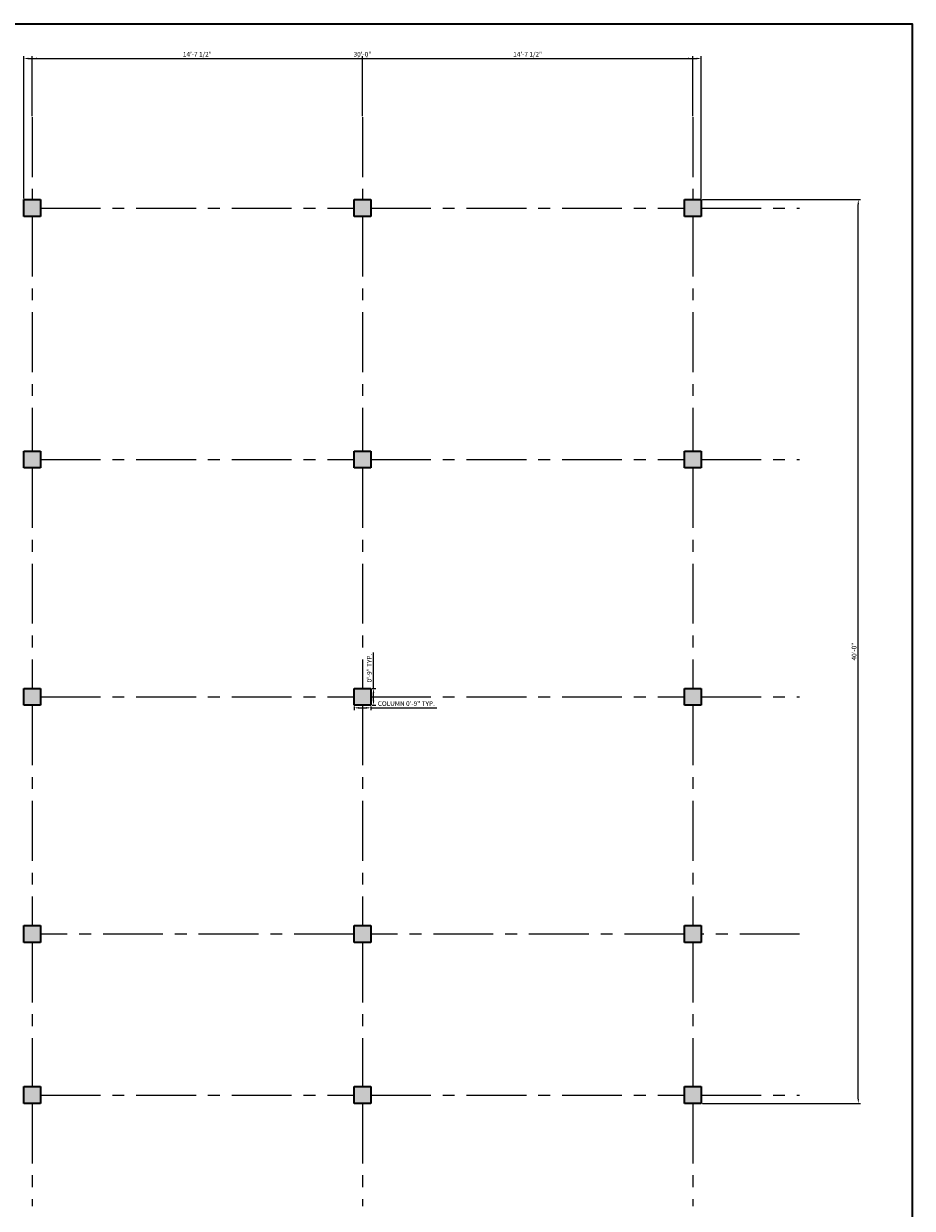
# Model space of a CAD drawing. Units: inches. Extents: x 2150 to 10686, y 1035 to 5077.
# Tile 4 of 12: x 2687 to 3159, y 1472 to 2101. Entities that reach past the tile are written whole.
import ezdxf

# ---------------------------------------------------------------- set-up
doc = ezdxf.new("R2010")
doc.units = ezdxf.units.IN
doc.linetypes.add('CENTER', pattern=[50.8, 31.75, -6.35, 6.35, -6.35])
for name, color, linetype, lineweight in [('A-ANNO-DIMS', 2, 'Continuous', 18), ('A-ANNO-TTLB', 7, 'Continuous', 35), ('A-COLS', 7, 'Continuous', 35), ('A-COLS-PATT', 8, 'Continuous', 13), ('A-GRID', 1, 'CENTER', 18)]:
    doc.layers.add(name, color=color, linetype=linetype, lineweight=lineweight)
doc.styles.get("Standard").update_dxf_attribs({"font": 'arial.ttf'})
doc.dimstyles.new('ISO-25', dxfattribs={"dimtxt": 2.5, "dimasz": 2.5, "dimexe": 1.25, "dimexo": 0.625, "dimtad": 1, "dimdec": 0, "dimlunit": 3, "dimtxsty": 'Standard', "dimcen": 2.5, "dimadec": 0, "dimazin": 0, "dimtfac": 1, "dimtdec": 0, "dimtmove": 0, "dimatfit": 3, "dimfxl": 1, "dimarcsym": 0})

# ---------------------------------------------------------------- blocks, each defined once
blk = doc.blocks.new('COL-SQUARE-9IN')
for p, q in [((0, 9), (9, 9)), ((0, 0), (0, 9)), ((9, 9), (9, 0)), ((9, 0), (0, 0))]:
    blk.add_line(p, q)
blk = doc.blocks.new('*D38')
at = {"layer": 'A-ANNO-DIMS', "color": 0, "lineweight": -2, "transparency": 16777216}
for p, q in [((2862.4, 1738.17), (2862.4, 1736.19)), ((2864.9, 1737.44), (2868.9, 1737.44)), ((2871.4, 1738.17), (2871.4, 1736.19)), ((2871.4, 1737.44), (2906.46, 1737.44))]:
    blk.add_line(p, q, dxfattribs=at)
at = {"layer": 'A-ANNO-DIMS', "color": 0, "transparency": 16777216}
for points in [[(2864.9, 1737.86), (2864.9, 1737.02), (2862.4, 1737.44)], [(2868.9, 1737.86), (2868.9, 1737.02), (2871.4, 1737.44)]]:
    blk.add_solid(points, dxfattribs=at)
at = {"layer": 'Defpoints', "color": 0, "transparency": 16777216}
for p in [(2862.4, 1738.79), (2871.4, 1738.79), (2871.4, 1737.44)]:
    blk.add_point(p, dxfattribs=at)
at = {"layer": 'A-ANNO-DIMS', "color": 0, "transparency": 16777216, "insert": (2890.18, 1739.36), "char_height": 2.5, "attachment_point": 5}
blk.add_mtext('COLUMN 0\'-9" TYP.', dxfattribs=at)
blk = doc.blocks.new('*D39')
at = {"layer": 'A-ANNO-DIMS', "color": 0, "lineweight": -2, "transparency": 16777216}
for p, q in [((2872.75, 1747.79), (2872.75, 1766.78)), ((2872.02, 1747.79), (2874, 1747.79)), ((2872.75, 1741.29), (2872.75, 1745.29)), ((2872.02, 1738.79), (2874, 1738.79))]:
    blk.add_line(p, q, dxfattribs=at)
at = {"layer": 'A-ANNO-DIMS', "color": 0, "transparency": 16777216}
for points in [[(2872.33, 1745.29), (2873.16, 1745.29), (2872.75, 1747.79)], [(2872.33, 1741.29), (2873.16, 1741.29), (2872.75, 1738.79)]]:
    blk.add_solid(points, dxfattribs=at)
at = {"layer": 'Defpoints', "color": 0, "transparency": 16777216}
for p in [(2871.4, 1747.79), (2872.75, 1747.79), (2871.4, 1738.79)]:
    blk.add_point(p, dxfattribs=at)
at = {"layer": 'A-ANNO-DIMS', "color": 0, "transparency": 16777216, "insert": (2870.85, 1758.54), "char_height": 2.5, "attachment_point": 5, "rotation": 90}
blk.add_mtext('0\'-9" TYP.', dxfattribs=at)
blk = doc.blocks.new('*D78')
at = {"layer": 'A-ANNO-DIMS', "color": 0, "lineweight": -2, "transparency": 16777216}
for p, q in [((2691.4, 2051.67), (2691.4, 2083.5)), ((2693.9, 2082.25), (2864.4, 2082.25)), ((2866.9, 2051.67), (2866.9, 2083.5))]:
    blk.add_line(p, q, dxfattribs=at)
at = {"layer": 'A-ANNO-DIMS', "color": 0, "transparency": 16777216}
for points in [[(2693.9, 2082.66), (2693.9, 2081.83), (2691.4, 2082.25)], [(2864.4, 2082.66), (2864.4, 2081.83), (2866.9, 2082.25)]]:
    blk.add_solid(points, dxfattribs=at)
at = {"layer": 'Defpoints', "color": 0, "transparency": 16777216}
for p in [(2866.9, 2082.25), (2691.4, 2051.05), (2866.9, 2051.05)]:
    blk.add_point(p, dxfattribs=at)
at = {"layer": 'A-ANNO-DIMS', "color": 0, "transparency": 16777216, "insert": (2779.15, 2084.16), "char_height": 2.5, "attachment_point": 5}
blk.add_mtext('14\'-7 1/2"', dxfattribs=at)
blk = doc.blocks.new('*D79')
at = {"layer": 'A-ANNO-DIMS', "color": 0, "lineweight": -2, "transparency": 16777216}
for p, q in [((2866.9, 2051.67), (2866.9, 2083.5)), ((2869.4, 2082.25), (3039.9, 2082.25)), ((3042.4, 2051.67), (3042.4, 2083.5))]:
    blk.add_line(p, q, dxfattribs=at)
at = {"layer": 'A-ANNO-DIMS', "color": 0, "transparency": 16777216}
for points in [[(2869.4, 2082.66), (2869.4, 2081.83), (2866.9, 2082.25)], [(3039.9, 2082.66), (3039.9, 2081.83), (3042.4, 2082.25)]]:
    blk.add_solid(points, dxfattribs=at)
at = {"layer": 'Defpoints', "color": 0, "transparency": 16777216}
for p in [(3042.4, 2082.25), (2866.9, 2051.05), (3042.4, 2051.05)]:
    blk.add_point(p, dxfattribs=at)
at = {"layer": 'A-ANNO-DIMS', "color": 0, "transparency": 16777216, "insert": (2954.65, 2084.16), "char_height": 2.5, "attachment_point": 5}
blk.add_mtext('14\'-7 1/2"', dxfattribs=at)
blk = doc.blocks.new('*D84')
at = {"layer": 'A-ANNO-DIMS', "color": 0, "lineweight": -2, "transparency": 16777216}
for p, q in [((2686.9, 2007.92), (2686.9, 2083.5)), ((2689.4, 2082.25), (3044.4, 2082.25)), ((3046.9, 2007.92), (3046.9, 2083.5))]:
    blk.add_line(p, q, dxfattribs=at)
at = {"layer": 'A-ANNO-DIMS', "color": 0, "transparency": 16777216}
for points in [[(2689.4, 2082.66), (2689.4, 2081.83), (2686.9, 2082.25)], [(3044.4, 2082.66), (3044.4, 2081.83), (3046.9, 2082.25)]]:
    blk.add_solid(points, dxfattribs=at)
at = {"layer": 'Defpoints', "color": 0, "transparency": 16777216}
for p in [(3046.9, 2082.25), (2686.9, 2007.29), (3046.9, 2007.29)]:
    blk.add_point(p, dxfattribs=at)
at = {"layer": 'A-ANNO-DIMS', "color": 0, "transparency": 16777216, "insert": (2866.9, 2084.15), "char_height": 2.5, "attachment_point": 5}
blk.add_mtext('30\'-0"', dxfattribs=at)
blk = doc.blocks.new('*D85')
at = {"layer": 'A-ANNO-DIMS', "color": 0, "lineweight": -2, "transparency": 16777216}
for p, q in [((3047.52, 2007.29), (3131.56, 2007.29)), ((3130.31, 1529.79), (3130.31, 2004.79)), ((3047.52, 1527.29), (3131.56, 1527.29))]:
    blk.add_line(p, q, dxfattribs=at)
at = {"layer": 'A-ANNO-DIMS', "color": 0, "transparency": 16777216}
for points in [[(3129.9, 2004.79), (3130.73, 2004.79), (3130.31, 2007.29)], [(3129.9, 1529.79), (3130.73, 1529.79), (3130.31, 1527.29)]]:
    blk.add_solid(points, dxfattribs=at)
at = {"layer": 'Defpoints', "color": 0, "transparency": 16777216}
for p in [(3046.9, 2007.29), (3130.31, 2007.29), (3046.9, 1527.29)]:
    blk.add_point(p, dxfattribs=at)
at = {"layer": 'A-ANNO-DIMS', "color": 0, "transparency": 16777216, "insert": (3128.41, 1767.29), "char_height": 2.5, "attachment_point": 5, "rotation": 90}
blk.add_mtext('40\'-0"', dxfattribs=at)

msp = doc.modelspace()

# ---------------------------------------------------------------- hatches: boundary and pattern name
at = {"layer": 'A-COLS-PATT'}
h = msp.add_hatch(color=256, dxfattribs=at)
h.dxf.hatch_style = 1
h.paths.add_polyline_path([(2695.9, 2007.29), (2686.9, 2007.29), (2686.9, 1998.29), (2695.9, 1998.29)])
h.paths.add_polyline_path([(2871.4, 2007.29), (2862.4, 2007.29), (2862.4, 1998.29), (2871.4, 1998.29)])
h.paths.add_polyline_path([(3046.9, 2007.29), (3037.9, 2007.29), (3037.9, 1998.29), (3046.9, 1998.29)])
h.paths.add_polyline_path([(2695.9, 1873.79), (2686.9, 1873.79), (2686.9, 1864.79), (2695.9, 1864.79)])
h.paths.add_polyline_path([(2871.4, 1873.79), (2862.4, 1873.79), (2862.4, 1864.79), (2871.4, 1864.79)])
h.paths.add_polyline_path([(3046.9, 1873.79), (3037.9, 1873.79), (3037.9, 1864.79), (3046.9, 1864.79)])
h.paths.add_polyline_path([(2695.9, 1747.79), (2686.9, 1747.79), (2686.9, 1738.79), (2695.9, 1738.79)])
h.paths.add_polyline_path([(2871.4, 1747.79), (2862.4, 1747.79), (2862.4, 1738.79), (2871.4, 1738.79)])
h.paths.add_polyline_path([(3046.9, 1747.79), (3037.9, 1747.79), (3037.9, 1738.79), (3046.9, 1738.79)])
h.paths.add_polyline_path([(2695.9, 1621.79), (2686.9, 1621.79), (2686.9, 1612.79), (2695.9, 1612.79)])
h.paths.add_polyline_path([(2871.4, 1621.79), (2862.4, 1621.79), (2862.4, 1612.79), (2871.4, 1612.79)])
h.paths.add_polyline_path([(3046.9, 1621.79), (3037.9, 1621.79), (3037.9, 1612.79), (3046.9, 1612.79)])
h.paths.add_polyline_path([(2695.9, 1536.29), (2686.9, 1536.29), (2686.9, 1527.29), (2695.9, 1527.29)])
h.paths.add_polyline_path([(2871.4, 1536.29), (2862.4, 1536.29), (2862.4, 1527.29), (2871.4, 1527.29)])
h.paths.add_polyline_path([(3046.9, 1536.29), (3037.9, 1536.29), (3037.9, 1527.29), (3046.9, 1527.29)])

# ---------------------------------------------------------------- linework, layer by layer
at = {"layer": 'A-ANNO-TTLB'}
msp.add_lwpolyline([(2149.86, 2100.72), (3159.01, 2100.72), (3159.01, 1034.91), (2149.86, 1034.91)], close=True, dxfattribs=at)
at = {"layer": 'A-GRID'}
for p, q in [((2691.4, 2051.05), (2691.4, 2007.29)), ((2866.9, 2051.05), (2866.9, 2007.29)), ((3042.4, 2051.05), (3042.4, 2007.29)), ((2695.9, 2002.79), (2862.4, 2002.79)), ((2871.4, 2002.79), (3037.9, 2002.79)), ((3046.9, 2002.79), (3099.11, 2002.79)), ((2691.4, 1998.29), (2691.4, 1873.79)), ((2866.9, 1998.29), (2866.9, 1873.79)), ((3042.4, 1998.29), (3042.4, 1873.79)), ((2695.9, 1869.29), (2862.4, 1869.29)), ((2871.4, 1869.29), (3037.9, 1869.29)), ((3046.9, 1869.29), (3099.11, 1869.29)), ((2691.4, 1864.79), (2691.4, 1747.79)), ((2866.9, 1864.79), (2866.9, 1747.79)), ((3042.4, 1864.79), (3042.4, 1747.79)), ((2695.9, 1743.29), (2862.4, 1743.29)), ((2871.4, 1743.29), (3037.9, 1743.29)), ((3046.9, 1743.29), (3099.11, 1743.29)), ((2691.4, 1738.79), (2691.4, 1621.79)), ((2866.9, 1738.79), (2866.9, 1621.79)), ((3042.4, 1738.79), (3042.4, 1621.79)), ((2862.4, 1617.29), (2695.9, 1617.29)), ((3037.9, 1617.29), (2871.4, 1617.29)), ((3099.11, 1617.29), (3046.9, 1617.29)), ((2691.4, 1612.79), (2691.4, 1536.29)), ((2866.9, 1612.79), (2866.9, 1536.29)), ((3042.4, 1612.79), (3042.4, 1536.29)), ((2695.9, 1531.79), (2862.4, 1531.79)), ((2871.4, 1531.79), (3037.9, 1531.79)), ((3046.9, 1531.79), (3099.11, 1531.79)), ((2691.4, 1527.29), (2691.4, 1472.77)), ((2866.9, 1527.29), (2866.9, 1472.77)), ((3042.4, 1527.29), (3042.4, 1472.77))]:
    msp.add_line(p, q, dxfattribs=at)

# ---------------------------------------------------------------- block references
at = {"layer": 'A-COLS'}
for p in [(2686.9, 1998.29), (2862.4, 1998.29), (3037.9, 1998.29), (2686.9, 1864.79), (2862.4, 1864.79), (3037.9, 1864.79), (2686.9, 1738.79), (2862.4, 1738.79), (3037.9, 1738.79), (2686.9, 1612.79), (2862.4, 1612.79), (3037.9, 1612.79), (2686.9, 1527.29), (2862.4, 1527.29), (3037.9, 1527.29)]:
    msp.add_blockref('COL-SQUARE-9IN', p, dxfattribs=at)

# ---------------------------------------------------------------- dimensions: what is measured, and where the dimension line sits
at = {"layer": 'A-ANNO-DIMS'}
for base, p1, p2, picture, middle in [((3046.9, 2082.25), (2686.9, 2007.29), (3046.9, 2007.29), '*D84', (2866.9, 2084.15)), ((2866.9, 2082.25), (2691.4, 2051.05), (2866.9, 2051.05), '*D78', (2779.15, 2084.16)), ((3042.4, 2082.25), (2866.9, 2051.05), (3042.4, 2051.05), '*D79', (2954.65, 2084.16))]:
    dim = msp.add_linear_dim(base=base, p1=p1, p2=p2, dimstyle='ISO-25', override={"dimdec": 1, "dimlfac": 1, "dimrnd": 0, "dimzin": 1, "dimdsep": 46, "dimlunit": 4, "dimfrac": 2}, dxfattribs=at)
    dim.commit()
    dim.dimension.update_dxf_attribs({"geometry": picture, "text_midpoint": middle})
dim = msp.add_linear_dim(base=(3130.31, 2007.29), p1=(3046.9, 1527.29), p2=(3046.9, 2007.29), angle=90, dimstyle='ISO-25', override={"dimdec": 1, "dimlfac": 1, "dimrnd": 0, "dimzin": 1, "dimdsep": 46, "dimlunit": 4, "dimfrac": 2}, dxfattribs=at)
dim.commit()
dim.dimension.update_dxf_attribs({"geometry": '*D85', "text_midpoint": (3128.41, 1767.29)})
dim = msp.add_linear_dim(base=(2872.75, 1747.79), p1=(2871.4, 1738.79), p2=(2871.4, 1747.79), angle=90, text='<> TYP.', dimstyle='ISO-25', override={"dimdec": 1, "dimlfac": 1, "dimrnd": 0, "dimzin": 1, "dimdsep": 46, "dimlunit": 4, "dimfrac": 2}, dxfattribs=at)
dim.commit()
dim.dimension.update_dxf_attribs({"geometry": '*D39', "text_midpoint": (2870.85, 1758.54)})
dim = msp.add_linear_dim(base=(2871.4, 1737.44), p1=(2862.4, 1738.79), p2=(2871.4, 1738.79), text='COLUMN <> TYP.', dimstyle='ISO-25', override={"dimdec": 1, "dimlfac": 1, "dimrnd": 0, "dimzin": 1, "dimdsep": 46, "dimlunit": 4, "dimfrac": 2}, dxfattribs=at)
dim.commit()
dim.dimension.update_dxf_attribs({"geometry": '*D38', "text_midpoint": (2890.18, 1739.36)})

doc.saveas('drawing.dxf')
